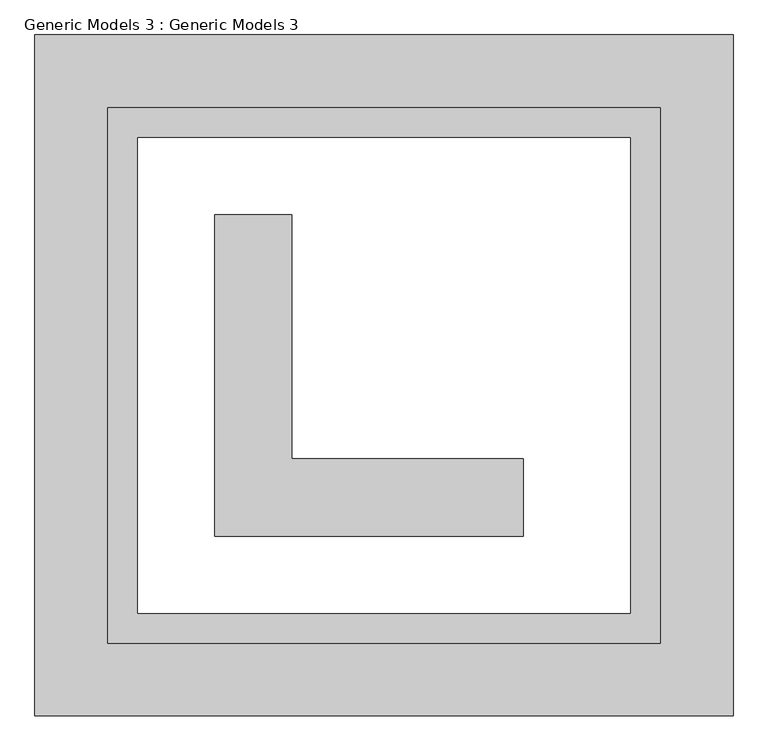
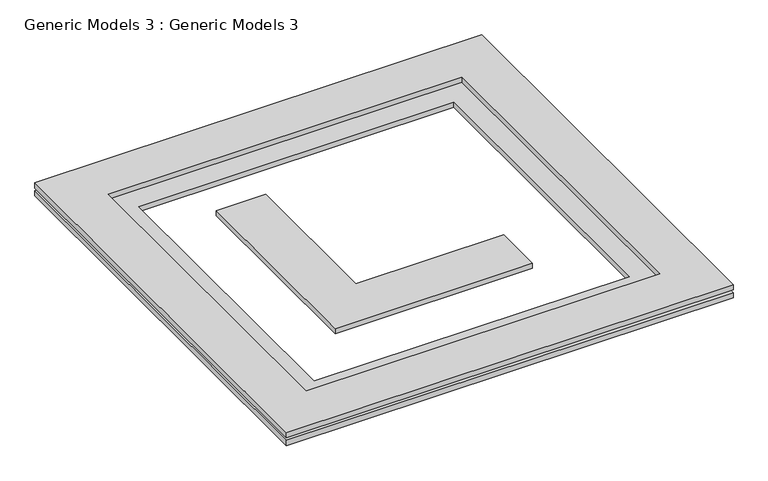
"""IFC4 building model written with IfcOpenShell, lengths in millimetres: proxy geometry, Generic Models 3 : Generic Models 3."""

from ifc_helpers import new_model, si_unit, frame, origin, place, context, project, spatial, polyline, outline, extrude, source, transform, mapped, element, save


def generic_models_3_generic_models_3_e47a0867(model_context):
    return source(origin(), model_context, "Body", "SweptSolid", [
        extrude(outline(polyline([(-12628.9002526, 11106.6128362), (-12171.7002526, 11106.6128362), (-12171.7002526, 9658.8128362), (-10800.1002526, 9658.8128362), (-10800.1002526, 9201.6128362), (-12628.9002526, 9201.6128362), (-12628.9002526, 11106.6128362)])), frame((0.0, 0.0, 2997.2), z_axis=(0.0, 0.0, 1.0), x_axis=(1.0, 0.0, 0.0)), (0.0, 0.0, 1.0), 50.8),
        extrude(outline(polyline([(-9555.5002526, 8134.8128362), (-13695.7002526, 8134.8128362), (-13695.7002526, 12173.4128362), (-9555.5002526, 12173.4128362), (-9555.5002526, 8134.8128362)]), holes=[polyline([(-10165.1002526, 8744.4128362), (-10165.1002526, 11563.8128362), (-13086.1002526, 11563.8128362), (-13086.1002526, 8744.4128362), (-10165.1002526, 8744.4128362)])]), frame((0.0, 0.0, 2921.0), z_axis=(0.0, 0.0, 1.0), x_axis=(1.0, 0.0, 0.0)), (0.0, 0.0, 1.0), 50.8),
        extrude(outline(polyline([(-9555.5002526, 8134.8128362), (-13695.7002526, 8134.8128362), (-13695.7002526, 12173.4128362), (-9555.5002526, 12173.4128362), (-9555.5002526, 8134.8128362)]), holes=[polyline([(-9987.3002526, 8566.6128362), (-9987.3002526, 11741.6128362), (-13263.9002526, 11741.6128362), (-13263.9002526, 8566.6128362), (-9987.3002526, 8566.6128362)])]), frame((0.0, 0.0, 2997.2), z_axis=(0.0, 0.0, 1.0), x_axis=(1.0, 0.0, 0.0)), (0.0, 0.0, 1.0), 50.8),
    ])


if __name__ == "__main__":
    model = new_model("IFC4")
    model_context = context("Model", 3, world=origin())
    ifc_project = project(units=[si_unit("LENGTHUNIT", "METRE", prefix="MILLI")], contexts=[model_context])
    site = spatial("IfcSite", under=ifc_project)
    building = spatial("IfcBuilding", under=site)
    placement = place(None, origin())
    generic_models_3_generic_models_3_shape = generic_models_3_generic_models_3_e47a0867(model_context)
    element("IfcBuildingElementProxy", 1, Name="Generic Models 3 : Generic Models 3", ObjectType="Generic Models 3 : Generic Models 3", at=placement, inside=building, context=model_context, shape_type="MappedRepresentation", body=[
        mapped(generic_models_3_generic_models_3_shape, transform((0.0, 0.0, 0.0), x_axis=(1.0, 0.0, 0.0), y_axis=(0.0, 1.0, 0.0), z_axis=(0.0, 0.0, 1.0))),
    ])
    save(model, "model.ifc")

# Revit data of these elements
# Element 1 (IfcBuildingElementProxy, "Generic Models 3 : Generic Models 3")
#   Materials on its faces: "Wall Material (1)", "1 light"
# Materials
#   "Wall Material (1)": colour RGB 80 80 80, transparency 0, Cost = 0
#   "1 light": colour RGB 242 242 242, transparency 1
